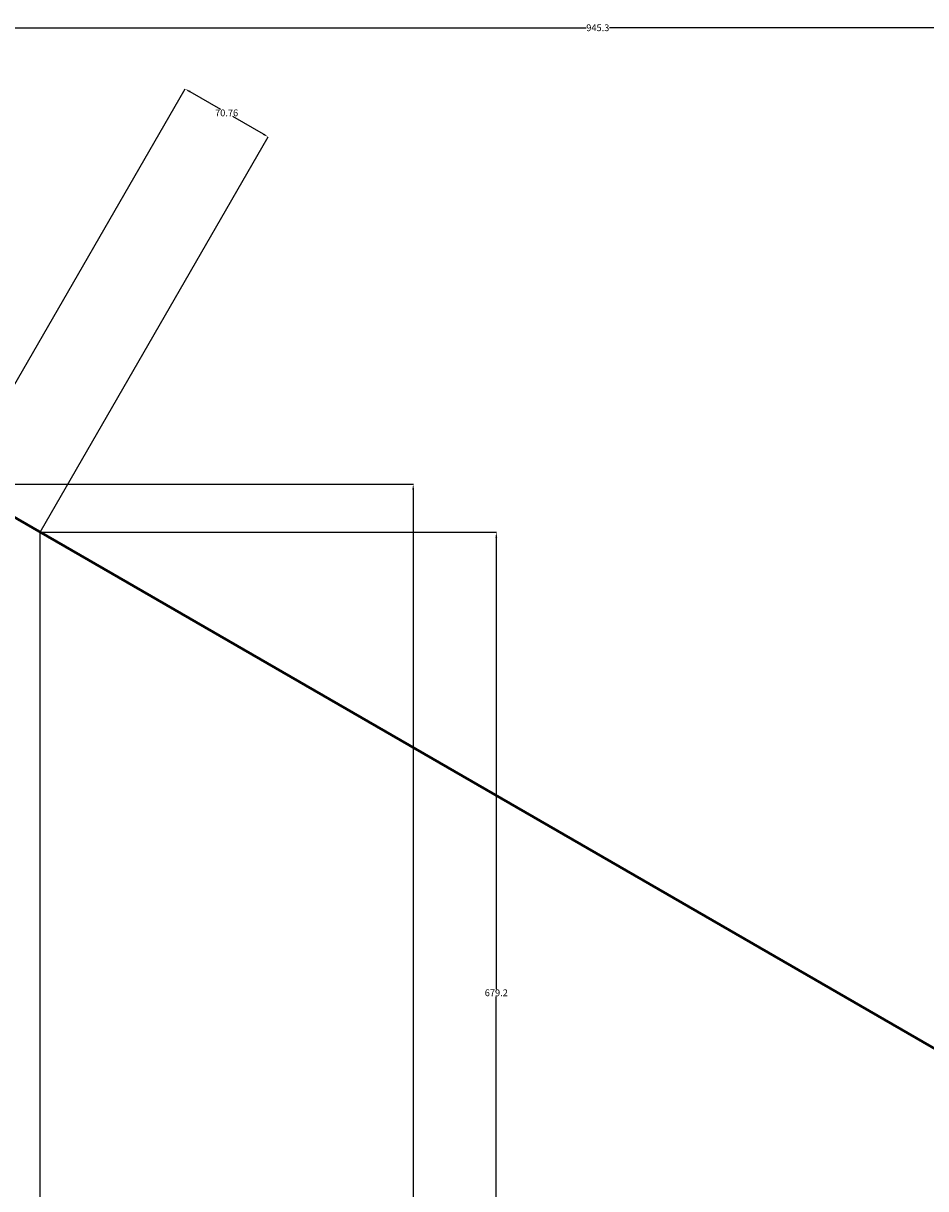
# Model space of a CAD drawing. Units: metres. Extents: x -2391 to 4922, y -635 to 4845.
# Tile 28 of 37: x 600 to 1265, y 3986 to 4845. Entities that reach past the tile are written whole.
import ezdxf

# ---------------------------------------------------------------- set-up
doc = ezdxf.new("R2010")
doc.units = ezdxf.units.M
doc.header["$MEASUREMENT"] = 0
for name, color, linetype, lineweight in [('A-ANNO-DIMS', 2, 'Continuous', 18), ('A-FLOR-FIXT', 3, 'Continuous', 25), ('A-WALL', 7, 'Continuous', 50)]:
    doc.layers.add(name, color=color, linetype=linetype, lineweight=lineweight)
doc.styles.get("Standard").update_dxf_attribs({"font": 'arial.ttf'})
doc.dimstyles.get("Standard").update_dxf_attribs({"dimtxt": 5, "dimasz": 4, "dimexe": 0.18, "dimexo": 0.0625, "dimgap": 0.09, "dimtad": 0, "dimtih": 1, "dimtoh": 1, "dimdec": 0, "dimzin": 0, "dimdsep": 46, "dimtxsty": 'Standard', "dimcen": 0.09, "dimadec": 0, "dimazin": 0, "dimtfac": 1, "dimtdec": 0, "dimtofl": 0, "dimtmove": 0, "dimatfit": 3, "dimfxl": 1, "dimtolj": 1, "dimtzin": 0, "dimarcsym": 0})

# ---------------------------------------------------------------- blocks, each defined once
blk = doc.blocks.new('*D11')
at = {"layer": 'A-ANNO-DIMS', "color": 0, "lineweight": -2, "transparency": 16777216}
for p, q in [((550.8, 4505.28), (887.42, 4505.28)), ((887.24, 4501.28), (887.24, 3317.92)), ((887.24, 2129.28), (887.24, 3312.63)), ((550.8, 2125.28), (887.42, 2125.28))]:
    blk.add_line(p, q, dxfattribs=at)
at = {"layer": 'A-ANNO-DIMS', "color": 0, "transparency": 16777216}
for points in [[(886.58, 4501.28), (887.91, 4501.28), (887.24, 4505.28)], [(886.58, 2129.28), (887.91, 2129.28), (887.24, 2125.28)]]:
    blk.add_solid(points, dxfattribs=at)
at = {"layer": 'Defpoints', "color": 0, "transparency": 16777216}
for p in [(550.74, 4505.28), (550.74, 2125.28), (887.24, 2125.28)]:
    blk.add_point(p, dxfattribs=at)
at = {"layer": 'A-ANNO-DIMS', "color": 0, "transparency": 16777216, "insert": (887.24, 3315.28), "char_height": 5, "attachment_point": 5}
blk.add_mtext('\\A1;2380', dxfattribs=at)
blk = doc.blocks.new('*D17')
at = {"layer": 'A-ANNO-DIMS', "color": 0, "lineweight": -2, "transparency": 16777216}
for p, q in [((550.74, 3005.34), (550.74, 4841.96)), ((554.74, 4841.78), (1014.86, 4841.78)), ((1492.03, 4841.78), (1031.91, 4841.78)), ((1496.03, 2662.52), (1496.03, 4841.96))]:
    blk.add_line(p, q, dxfattribs=at)
at = {"layer": 'A-ANNO-DIMS', "color": 0, "transparency": 16777216}
for points in [[(554.74, 4842.44), (554.74, 4841.11), (550.74, 4841.78)], [(1492.03, 4842.44), (1492.03, 4841.11), (1496.03, 4841.78)]]:
    blk.add_solid(points, dxfattribs=at)
at = {"layer": 'Defpoints', "color": 0, "transparency": 16777216}
for p in [(1496.03, 4841.78), (550.74, 3005.28), (1496.03, 2662.46)]:
    blk.add_point(p, dxfattribs=at)
at = {"layer": 'A-ANNO-DIMS', "color": 0, "transparency": 16777216, "insert": (1023.39, 4841.78), "char_height": 5, "attachment_point": 5}
blk.add_mtext('\\A1;945.3', dxfattribs=at)
blk = doc.blocks.new('*D32')
at = {"layer": 'A-ANNO-DIMS', "color": 0, "lineweight": -2, "transparency": 16777216}
for p, q in [((612.09, 4469.9), (948.7, 4469.9)), ((948.52, 4465.9), (948.52, 4132.92)), ((948.52, 3794.66), (948.52, 4127.63)), ((612.09, 3790.66), (948.7, 3790.66))]:
    blk.add_line(p, q, dxfattribs=at)
at = {"layer": 'A-ANNO-DIMS', "color": 0, "transparency": 16777216}
for points in [[(947.86, 4465.9), (949.19, 4465.9), (948.52, 4469.9)], [(947.86, 3794.66), (949.19, 3794.66), (948.52, 3790.66)]]:
    blk.add_solid(points, dxfattribs=at)
at = {"layer": 'Defpoints', "color": 0, "transparency": 16777216}
for p in [(612.02, 4469.9), (612.02, 3790.66), (948.52, 3790.66)]:
    blk.add_point(p, dxfattribs=at)
at = {"layer": 'A-ANNO-DIMS', "color": 0, "transparency": 16777216, "insert": (948.52, 4130.28), "char_height": 5, "attachment_point": 5}
blk.add_mtext('\\A1;679.2', dxfattribs=at)
blk = doc.blocks.new('*D34')
at = {"layer": 'A-ANNO-DIMS', "color": 0, "lineweight": -2, "transparency": 16777216}
for p, q in [((550.77, 4505.33), (719.08, 4796.85)), ((722.46, 4794.69), (745.06, 4781.65)), ((776.81, 4763.31), (754.21, 4776.36)), ((612.05, 4469.95), (780.36, 4761.47))]:
    blk.add_line(p, q, dxfattribs=at)
at = {"layer": 'A-ANNO-DIMS', "color": 0, "transparency": 16777216}
for points in [[(722.79, 4795.27), (722.12, 4794.12), (718.99, 4796.69)], [(777.14, 4763.89), (776.48, 4762.74), (780.27, 4761.31)]]:
    blk.add_solid(points, dxfattribs=at)
at = {"layer": 'Defpoints', "color": 0, "transparency": 16777216}
for p in [(780.27, 4761.31), (550.74, 4505.28), (612.02, 4469.9)]:
    blk.add_point(p, dxfattribs=at)
at = {"layer": 'A-ANNO-DIMS', "color": 0, "transparency": 16777216, "insert": (749.63, 4779), "char_height": 5, "attachment_point": 5}
blk.add_mtext('\\A1;70.76', dxfattribs=at)

msp = doc.modelspace()

# ---------------------------------------------------------------- linework, layer by layer
at = {"layer": 'A-FLOR-FIXT'}
msp.add_line((612.0233, 3719.8954), (612.0233, 4469.8954), dxfattribs=at)
at = {"layer": 'A-WALL'}
msp.add_line((550.7419, 4505.2763), (3607.8116, 2740.2763), dxfattribs=at)

# ---------------------------------------------------------------- dimensions: what is measured, and where the dimension line sits
at = {"layer": 'A-ANNO-DIMS'}
dim = msp.add_linear_dim(base=(1496.0309, 4841.7763), p1=(550.7419, 3005.2763), p2=(1496.0309, 2662.4566), dimstyle='Standard', override={"dimdec": 1, "dimlfac": 1, "dimrnd": 0, "dimzin": 0, "dimdsep": 46, "dimlunit": 2}, dxfattribs=at)
dim.commit()
dim.dimension.update_dxf_attribs({"geometry": '*D17', "text_midpoint": (1023.3864, 4841.7763)})
for base, p1, p2, angle, override, picture, middle in [((780.2733, 4761.313), (550.7419, 4505.2763), (612.0233, 4469.8954), 330, {"dimdec": 2, "dimlfac": 1, "dimrnd": 0, "dimzin": 0, "dimdsep": 46, "dimlunit": 2}, '*D34', (749.6326, 4779.0034)), ((887.2419, 2125.2763), (550.7419, 4505.2763), (550.7419, 2125.2763), 270, {"dimdec": 0, "dimlfac": 1, "dimrnd": 0, "dimzin": 0, "dimdsep": 46, "dimlunit": 2}, '*D11', (887.2419, 3315.2763)), ((948.5233, 3790.6571), (612.0233, 4469.8954), (612.0233, 3790.6571), 270, {"dimdec": 1, "dimlfac": 1, "dimrnd": 0, "dimzin": 0, "dimdsep": 46, "dimlunit": 2}, '*D32', (948.5233, 4130.2763))]:
    dim = msp.add_linear_dim(base=base, p1=p1, p2=p2, angle=angle, dimstyle='Standard', override=override, dxfattribs=at)
    dim.commit()
    dim.dimension.update_dxf_attribs({"geometry": picture, "text_midpoint": middle})

doc.saveas('drawing.dxf')
